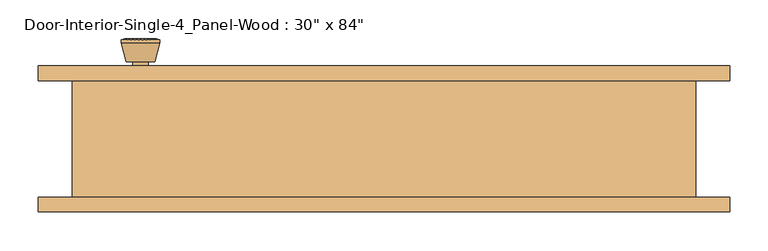
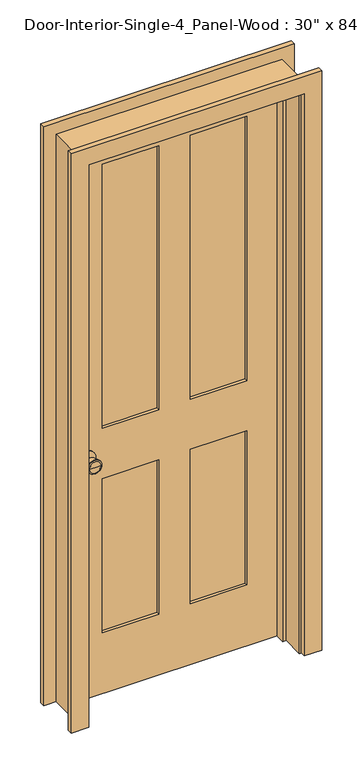
"""IFC4 building model written with IfcOpenShell, lengths in millimetres: door geometry."""

from ifc_helpers import new_model, si_unit, point, frame, frame_2d, origin, place, context, project, spatial, polyline, circle_curve, trimmed, segment, composite_curve, outline, extrude, faceted_brep, source, transform, mapped, element, save
from ifc_brep_helpers import plane_surface, cylinder_surface, revolved_surface, advanced_brep


def door_a7370db0(model_context):
    return source(origin(), model_context, "Body", "SolidModel", [
        advanced_brep(
        [(-317.5, 32.1, 914.4), (-307.5, 32.1, 914.4), (-327.5, 32.1, 914.4), (-297.0241324, -16.9, 914.4), (-317.5, -16.9, 914.4), (-337.9758676, -16.9, 914.4), (-292.5, -15.0721319, 914.4), (-342.5, -15.0721319, 914.4), (-292.5, -11.6084537, 914.4), (-342.5, -11.6084537, 914.4), (-298.863764, 13.1, 914.4), (-336.136236, 13.1, 914.4), (-307.5, 13.1, 914.4), (-327.5, 13.1, 914.4)],
        [
            (0, 1),
            (1, 2, circle_curve(frame((-317.5, 32.1, 914.4), z_axis=(0.0, 1.0, 0.0), x_axis=(-1.0, 0.0, 0.0)), 10.0)),
            (2, 0),
            (2, 1, circle_curve(frame((-317.5, 32.1, 914.4), z_axis=(0.0, 1.0, 0.0), x_axis=(-1.0, 0.0, 0.0)), 10.0)),
            (3, 4),
            (4, 5),
            (5, 3, circle_curve(frame((-317.5, -16.9, 914.4), z_axis=(0.0, -1.0, 0.0), x_axis=(-1.0, 0.0, 0.0)), 20.4758676)),
            (3, 5, circle_curve(frame((-317.5, -16.9, 914.4), z_axis=(0.0, -1.0, 0.0), x_axis=(-1.0, 0.0, 0.0)), 20.4758676)),
            (6, 3),
            (5, 7),
            (7, 6, circle_curve(frame((-317.5, -15.0721319, 914.4), z_axis=(0.0, -1.0, 0.0), x_axis=(-1.0, 0.0, 0.0)), 25.0)),
            (6, 7, circle_curve(frame((-317.5, -15.0721319, 914.4), z_axis=(0.0, -1.0, 0.0), x_axis=(-1.0, 0.0, 0.0)), 25.0)),
            (8, 6),
            (7, 9),
            (9, 8, circle_curve(frame((-317.5, -11.6084537, 914.4), z_axis=(0.0, -1.0, 0.0), x_axis=(-1.0, 0.0, 0.0)), 25.0)),
            (8, 9, circle_curve(frame((-317.5, -11.6084537, 914.4), z_axis=(0.0, -1.0, 0.0), x_axis=(-1.0, 0.0, 0.0)), 25.0)),
            (10, 8),
            (9, 11),
            (11, 10, circle_curve(frame((-317.5, 13.1, 914.4), z_axis=(0.0, -1.0, 0.0), x_axis=(-1.0, 0.0, 0.0)), 18.636236)),
            (10, 11, circle_curve(frame((-317.5, 13.1, 914.4), z_axis=(0.0, -1.0, 0.0), x_axis=(-1.0, 0.0, 0.0)), 18.636236)),
            (12, 10),
            (11, 13),
            (13, 12, circle_curve(frame((-317.5, 13.1, 914.4), z_axis=(0.0, -1.0, 0.0), x_axis=(-1.0, 0.0, 0.0)), 10.0)),
            (12, 13, circle_curve(frame((-317.5, 13.1, 914.4), z_axis=(0.0, -1.0, 0.0), x_axis=(-1.0, 0.0, 0.0)), 10.0)),
            (1, 12),
            (13, 2),
        ],
        [
            plane_surface(frame((-317.5, 32.1, 914.4), z_axis=(0.0, 1.0, 0.0), x_axis=(-1.0, 0.0, 0.0))),
            plane_surface(frame((-317.5, -16.9, 914.4), z_axis=(0.0, -1.0, 0.0), x_axis=(-1.0, 0.0, 0.0))),
            revolved_surface(polyline([(-337.9758676, -16.9, 914.4), (-342.5, -15.0721319, 914.4)]), (-317.5, 32.1, 914.4), (0.0, 1.0, 0.0)),
            cylinder_surface(frame((-317.5, 32.1, 914.4), z_axis=(0.0, 1.0, 0.0), x_axis=(-1.0, 0.0, 0.0)), 25.0),
            revolved_surface(polyline([(-342.5, -11.6084537, 914.4), (-336.136236, 13.1, 914.4)]), (-317.5, 32.1, 914.4), (0.0, 1.0, 0.0)),
            plane_surface(frame((-317.5, 13.1, 914.4), z_axis=(0.0, 1.0, 0.0), x_axis=(-1.0, 0.0, 0.0))),
            cylinder_surface(frame((-317.5, 32.1, 914.4), z_axis=(0.0, 1.0, 0.0), x_axis=(-1.0, 0.0, 0.0)), 10.0),
        ],
        [
            (0, [[1, 2, 3]]),
            (0, [[-3, 4, -1]]),
            (1, [[5, 6, 7]]),
            (1, [[-6, -5, 8]]),
            (2, [[9, -7, 10, 11]]),
            (2, [[-10, -8, -9, 12]]),
            (3, [[13, -11, 14, 15]]),
            (3, [[-14, -12, -13, 16]]),
            (4, [[17, -15, 18, 19]]),
            (4, [[-18, -16, -17, 20]]),
            (5, [[21, -19, 22, 23]]),
            (5, [[-22, -20, -21, 24]]),
            (6, [[25, -23, 26, -2]]),
            (6, [[-26, -24, -25, -4]]),
        ],
    ),
        extrude(outline(composite_curve([segment(trimmed(circle_curve(frame_2d((914.4, -317.5)), 30.0), [point((914.4, -347.5))], [point((914.4, -287.5))], False, "CARTESIAN"), True, "CONTINUOUS"), segment(trimmed(circle_curve(frame_2d((914.4, -317.5)), 30.0), [point((914.4, -287.5))], [point((914.4, -347.5))], False, "CARTESIAN"), True, "CONTINUOUS")], self_intersect=False)), frame((0.0, 32.1, 0.0), z_axis=(0.0, 1.0, 0.0), x_axis=(0.0, 0.0, 1.0)), (0.0, 0.0, 1.0), 6.0),
        advanced_brep(
        [(-317.5, 79.025, 914.4), (-327.5, 79.025, 914.4), (-307.5, 79.025, 914.4), (-297.0241324, 128.025, 914.4), (-337.9758676, 128.025, 914.4), (-317.5, 128.025, 914.4), (-292.5, 126.1971319, 914.4), (-342.5, 126.1971319, 914.4), (-292.5, 122.7334537, 914.4), (-342.5, 122.7334537, 914.4), (-298.863764, 98.025, 914.4), (-336.136236, 98.025, 914.4), (-307.5, 98.025, 914.4), (-327.5, 98.025, 914.4)],
        [
            (0, 1),
            (1, 2, circle_curve(frame((-317.5, 79.025, 914.4), z_axis=(0.0, -1.0, 0.0), x_axis=(-1.0, 0.0, 0.0)), 10.0)),
            (2, 0),
            (2, 1, circle_curve(frame((-317.5, 79.025, 914.4), z_axis=(0.0, -1.0, 0.0), x_axis=(-1.0, 0.0, 0.0)), 10.0)),
            (3, 4, circle_curve(frame((-317.5, 128.025, 914.4), z_axis=(0.0, 1.0, 0.0), x_axis=(-1.0, 0.0, 0.0)), 20.4758676)),
            (4, 5),
            (5, 3),
            (4, 3, circle_curve(frame((-317.5, 128.025, 914.4), z_axis=(0.0, 1.0, 0.0), x_axis=(-1.0, 0.0, 0.0)), 20.4758676)),
            (6, 7, circle_curve(frame((-317.5, 126.1971319, 914.4), z_axis=(0.0, 1.0, 0.0), x_axis=(-1.0, 0.0, 0.0)), 25.0)),
            (7, 4),
            (3, 6),
            (7, 6, circle_curve(frame((-317.5, 126.1971319, 914.4), z_axis=(0.0, 1.0, 0.0), x_axis=(-1.0, 0.0, 0.0)), 25.0)),
            (8, 9, circle_curve(frame((-317.5, 122.7334537, 914.4), z_axis=(0.0, 1.0, 0.0), x_axis=(-1.0, 0.0, 0.0)), 25.0)),
            (9, 7),
            (6, 8),
            (9, 8, circle_curve(frame((-317.5, 122.7334537, 914.4), z_axis=(0.0, 1.0, 0.0), x_axis=(-1.0, 0.0, 0.0)), 25.0)),
            (10, 11, circle_curve(frame((-317.5, 98.025, 914.4), z_axis=(0.0, 1.0, 0.0), x_axis=(-1.0, 0.0, 0.0)), 18.636236)),
            (11, 9),
            (8, 10),
            (11, 10, circle_curve(frame((-317.5, 98.025, 914.4), z_axis=(0.0, 1.0, 0.0), x_axis=(-1.0, 0.0, 0.0)), 18.636236)),
            (12, 13, circle_curve(frame((-317.5, 98.025, 914.4), z_axis=(0.0, 1.0, 0.0), x_axis=(-1.0, 0.0, 0.0)), 10.0)),
            (13, 11),
            (10, 12),
            (13, 12, circle_curve(frame((-317.5, 98.025, 914.4), z_axis=(0.0, 1.0, 0.0), x_axis=(-1.0, 0.0, 0.0)), 10.0)),
            (1, 13),
            (12, 2),
        ],
        [
            plane_surface(frame((-317.5, 79.025, 914.4), z_axis=(0.0, -1.0, 0.0), x_axis=(-1.0, 0.0, 0.0))),
            plane_surface(frame((-317.5, 128.025, 914.4), z_axis=(0.0, 1.0, 0.0), x_axis=(-1.0, 0.0, 0.0))),
            revolved_surface(polyline([(-337.9758676, 128.025, 914.4), (-342.5, 126.1971319, 914.4)]), (-317.5, 79.025, 914.4), (0.0, -1.0, 0.0)),
            cylinder_surface(frame((-317.5, 79.025, 914.4), z_axis=(0.0, -1.0, 0.0), x_axis=(-1.0, 0.0, 0.0)), 25.0),
            revolved_surface(polyline([(-342.5, 122.7334537, 914.4), (-336.136236, 98.025, 914.4)]), (-317.5, 79.025, 914.4), (0.0, -1.0, 0.0)),
            plane_surface(frame((-317.5, 98.025, 914.4), z_axis=(0.0, -1.0, 0.0), x_axis=(-1.0, 0.0, 0.0))),
            cylinder_surface(frame((-317.5, 79.025, 914.4), z_axis=(0.0, -1.0, 0.0), x_axis=(-1.0, 0.0, 0.0)), 10.0),
        ],
        [
            (0, [[1, 2, 3]]),
            (0, [[-3, 4, -1]]),
            (1, [[5, 6, 7]]),
            (1, [[8, -7, -6]]),
            (2, [[9, 10, -5, 11]]),
            (2, [[12, -11, -8, -10]]),
            (3, [[13, 14, -9, 15]]),
            (3, [[16, -15, -12, -14]]),
            (4, [[17, 18, -13, 19]]),
            (4, [[20, -19, -16, -18]]),
            (5, [[21, 22, -17, 23]]),
            (5, [[24, -23, -20, -22]]),
            (6, [[-2, 25, -21, 26]]),
            (6, [[-4, -26, -24, -25]]),
        ],
    ),
        extrude(outline(composite_curve([segment(trimmed(circle_curve(frame_2d((914.4, -317.5)), 30.0), [point((914.4, -347.5))], [point((914.4, -287.5))], False, "CARTESIAN"), True, "CONTINUOUS"), segment(trimmed(circle_curve(frame_2d((914.4, -317.5)), 30.0), [point((914.4, -287.5))], [point((914.4, -347.5))], False, "CARTESIAN"), True, "CONTINUOUS")], self_intersect=False)), frame((0.0, 73.025, 0.0), z_axis=(0.0, 1.0, 0.0), x_axis=(0.0, 0.0, 1.0)), (0.0, 0.0, 1.0), 6.0),
        extrude(outline(polyline([(260.35, 49.7416667), (57.15, 49.7416667), (57.15, 61.3833333), (260.35, 61.3833333), (260.35, 49.7416667)])), frame((0.0, 0.0, 1009.65), z_axis=(0.0, 0.0, 1.0), x_axis=(1.0, 0.0, 0.0)), (0.0, 0.0, 1.0), 1004.8875),
        extrude(outline(polyline([(-57.15, 49.7416667), (-260.35, 49.7416667), (-260.35, 61.3833333), (-57.15, 61.3833333), (-57.15, 49.7416667)])), frame((0.0, 0.0, 1009.65), z_axis=(0.0, 0.0, 1.0), x_axis=(1.0, 0.0, 0.0)), (0.0, 0.0, 1.0), 1004.8875),
        extrude(outline(polyline([(260.35, 49.7416667), (57.15, 49.7416667), (57.15, 61.3833333), (260.35, 61.3833333), (260.35, 49.7416667)])), frame((0.0, 0.0, 231.775), z_axis=(0.0, 0.0, 1.0), x_axis=(1.0, 0.0, 0.0)), (0.0, 0.0, 1.0), 587.375),
        extrude(outline(polyline([(-57.15, 49.7416667), (-260.35, 49.7416667), (-260.35, 61.3833333), (-57.15, 61.3833333), (-57.15, 49.7416667)])), frame((0.0, 0.0, 231.775), z_axis=(0.0, 0.0, 1.0), x_axis=(1.0, 0.0, 0.0)), (0.0, 0.0, 1.0), 587.375),
        extrude(outline(polyline([(2133.6, -381.0), (0.0, -381.0), (0.0, 381.0), (2133.6, 381.0), (2133.6, -381.0)]), holes=[polyline([(2014.5375, 57.15), (2014.5375, 260.35), (1009.65, 260.35), (1009.65, 57.15), (2014.5375, 57.15)]), polyline([(1009.65, -57.15), (1009.65, -260.35), (2014.5375, -260.35), (2014.5375, -57.15), (1009.65, -57.15)]), polyline([(819.15, 57.15), (819.15, 260.35), (231.775, 260.35), (231.775, 57.15), (819.15, 57.15)]), polyline([(231.775, -57.15), (231.775, -260.35), (819.15, -260.35), (819.15, -57.15), (231.775, -57.15)])]), frame((0.0, 38.1, 0.0), z_axis=(0.0, 1.0, 0.0), x_axis=(0.0, 0.0, 1.0)), (0.0, 0.0, 1.0), 34.925),
        faceted_brep([(406.4, 73.025, 0.0), (406.4, -79.375, 0.0), (381.0, -79.375, 0.0), (381.0, 3.175, 0.0), (368.3, 3.175, 0.0), (368.3, 38.1, 0.0), (381.0, 38.1, 0.0), (381.0, 73.025, 0.0), (406.4, 73.025, 2159.0), (406.4, -79.375, 2159.0), (-406.4, -79.375, 2159.0), (-406.4, -79.375, 0.0), (-381.0, -79.375, 0.0), (-381.0, -79.375, 2133.6), (381.0, -79.375, 2133.6), (381.0, 3.175, 2133.6), (-381.0, 3.175, 2133.6), (-381.0, 3.175, 0.0), (-368.3, 3.175, 0.0), (-368.3, 3.175, 2120.9), (368.3, 3.175, 2120.9), (368.3, 38.1, 2120.9), (-368.3, 38.1, 2120.9), (-368.3, 38.1, 0.0), (-381.0, 38.1, 0.0), (-381.0, 38.1, 2133.6), (381.0, 38.1, 2133.6), (381.0, 73.025, 2133.6), (-381.0, 73.025, 2133.6), (-381.0, 73.025, 0.0), (-406.4, 73.025, 0.0), (-406.4, 73.025, 2159.0)], [[[0, 1, 2, 3, 4, 5, 6, 7]], [[1, 0, 8, 9]], [[2, 1, 9, 10, 11, 12, 13, 14]], [[3, 2, 14, 15]], [[4, 3, 15, 16, 17, 18, 19, 20]], [[5, 4, 20, 21]], [[6, 5, 21, 22, 23, 24, 25, 26]], [[7, 6, 26, 27]], [[0, 7, 27, 28, 29, 30, 31, 8]], [[9, 8, 31, 10]], [[15, 14, 13, 16]], [[21, 20, 19, 22]], [[27, 26, 25, 28]], [[30, 29, 24, 23, 18, 17, 12, 11]], [[10, 31, 30, 11]], [[16, 13, 12, 17]], [[22, 19, 18, 23]], [[28, 25, 24, 29]]]),
        extrude(outline(polyline([(0.0, 387.35), (0.0, 450.85), (2203.45, 450.85), (2203.45, -450.85), (0.0, -450.85), (0.0, -387.35), (2139.95, -387.35), (2139.95, 387.35), (0.0, 387.35)])), frame((0.0, -98.425, 0.0), z_axis=(0.0, 1.0, 0.0), x_axis=(0.0, 0.0, 1.0)), (0.0, 0.0, 1.0), 19.05),
        extrude(outline(polyline([(0.0, 387.35), (0.0, 450.85), (2203.45, 450.85), (2203.45, -450.85), (0.0, -450.85), (0.0, -387.35), (2139.95, -387.35), (2139.95, 387.35), (0.0, 387.35)])), frame((0.0, 73.025, 0.0), z_axis=(0.0, 1.0, 0.0), x_axis=(0.0, 0.0, 1.0)), (0.0, 0.0, 1.0), 19.05),
    ])


if __name__ == "__main__":
    model = new_model("IFC4")
    model_context = context("Model", 3, world=origin())
    ifc_project = project(units=[si_unit("LENGTHUNIT", "METRE", prefix="MILLI")], contexts=[model_context])
    site = spatial("IfcSite", under=ifc_project)
    building = spatial("IfcBuilding", under=site)
    placement = place(None, origin())
    door_shape = door_a7370db0(model_context)
    element("IfcDoor", 1, ObjectType="Door-Interior-Single-4_Panel-Wood : 30\" x 84\"", at=placement, inside=building, context=model_context, shape_type="MappedRepresentation", body=[
        mapped(door_shape, transform((0.0, 0.0, 0.0), x_axis=(1.0, 0.0, 0.0), y_axis=(0.0, 1.0, 0.0), z_axis=(0.0, 0.0, 1.0))),
    ])
    save(model, "model.ifc")

# Revit data of these elements
# Type "Door-Interior-Single-4_Panel-Wood : 30\" x 84\""
#   Type Mark = "9"
#   Assembly Code = "C1020300"
#   Analytic Construction = "Wooden"
#   Top Rail = 0' - 4 11/16"
#   Thickness = 0' - 1 3/8"
#   Thermal Resistance (R) = 2.5876 (h·ft²·°F)/BTU
#   Swing Angle [instance default] = 90.00°
#   Stiles = 0' - 4 3/4"
#   Rough Width = 2' - 8"
#   Rough Height = 7' - 1"
#   Mullion = 0' - 4 1/2"
#   Lock Rail = 0' - 7 1/2"
#   Height = 7' - 0"
#   Width = 2' - 6"
#   Heat Transfer Coefficient (U) = 0.3865 BTU/(h·ft²·°F)
#   Bottom Rail = 0' - 9 1/8"
#   Trim Material = Cherry
#   Panel Material = Cherry
#   Frame Material = Cherry
#   Door Handle Material = Aluminum
#   Visual Light Transmittance = 0
#   Solar Heat Gain Coefficient = 0
#   Wall Closure = (empty or 0)
#   Function = (empty or 0)
# Element 1 (IfcDoor, "Door-Interior-Single-4_Panel-Wood : 30\" x 84\"")
#   Materials on its faces: "Cherry", "Aluminum"
# Materials
#   "Cherry": class "Wood", colour RGB 226 177 128, transparency 0, Description = "Prunus Serotina", Cost = 0
#   "Aluminum": class "Metal", colour RGB 247 247 247, transparency 0, Description = "Aluminum 6061", Cost = 0
